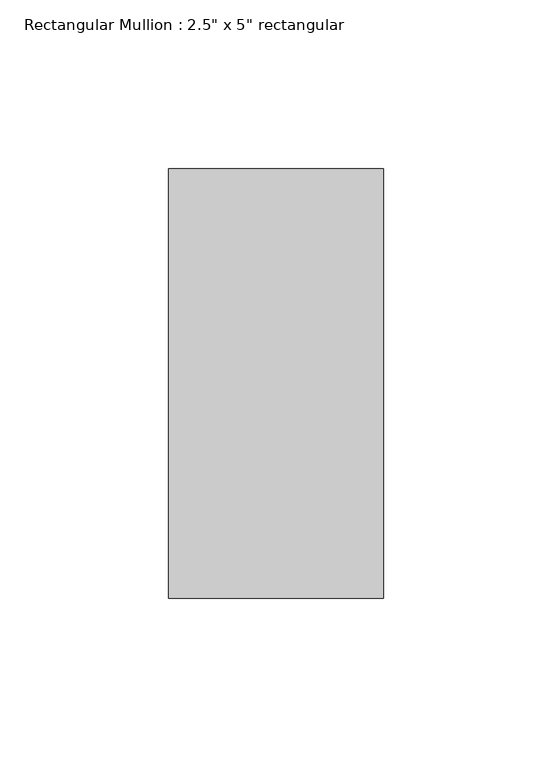
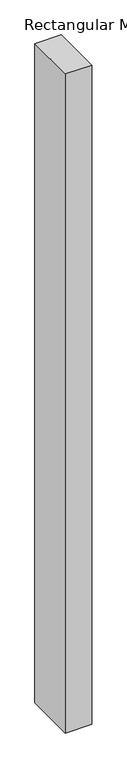
"""IFC4 building model written with IfcOpenShell, lengths in millimetres: member geometry."""

from ifc_helpers import new_model, si_unit, frame, origin, place, context, project, spatial, polyline, outline, extrude, source, transform, mapped, element, save


def member_78adf786(model_context):
    return source(origin(), model_context, "Body", "SweptSolid", [
        extrude(outline(polyline([(0.0, 63.5), (0.0, -63.5), (-63.5, -63.5), (-63.5, 63.5), (0.0, 63.5)])), frame((0.0, 0.0, -1681.1349385), z_axis=(0.0, 0.0, 1.0), x_axis=(1.0, 0.0, 0.0)), (0.0, 0.0, 1.0), 1681.1349385),
    ])


if __name__ == "__main__":
    model = new_model("IFC4")
    model_context = context("Model", 3, world=origin())
    ifc_project = project(units=[si_unit("LENGTHUNIT", "METRE", prefix="MILLI")], contexts=[model_context])
    site = spatial("IfcSite", under=ifc_project)
    building = spatial("IfcBuilding", under=site)
    placement = place(None, origin())
    member_shape = member_78adf786(model_context)
    element("IfcMember", 1, ObjectType="Rectangular Mullion : 2.5\" x 5\" rectangular", at=placement, inside=building, context=model_context, shape_type="MappedRepresentation", body=[
        mapped(member_shape, transform((0.0, 0.0, 0.0), x_axis=(1.0, 0.0, 0.0), y_axis=(0.0, 1.0, 0.0), z_axis=(0.0, 0.0, 1.0))),
    ])
    save(model, "model.ifc")

# Revit data of these elements
# Type "Rectangular Mullion : 2.5\" x 5\" rectangular"
#   built-in parameter 1007304 = 0.416667 (stored number, unit not read)
#   built-in parameter 1007301 = 0.104167 (stored number, unit not read)
#   built-in parameter 1007300 = 0.104167 (stored number, unit not read)
# Element 1 (IfcMember, "Rectangular Mullion : 2.5\" x 5\" rectangular")
#   Materials on its faces: "Aluminum"
# Materials
#   "Aluminum": class "Metal", colour RGB 247 247 247, transparency 0, Description = "Aluminum 6061", Cost = 0
